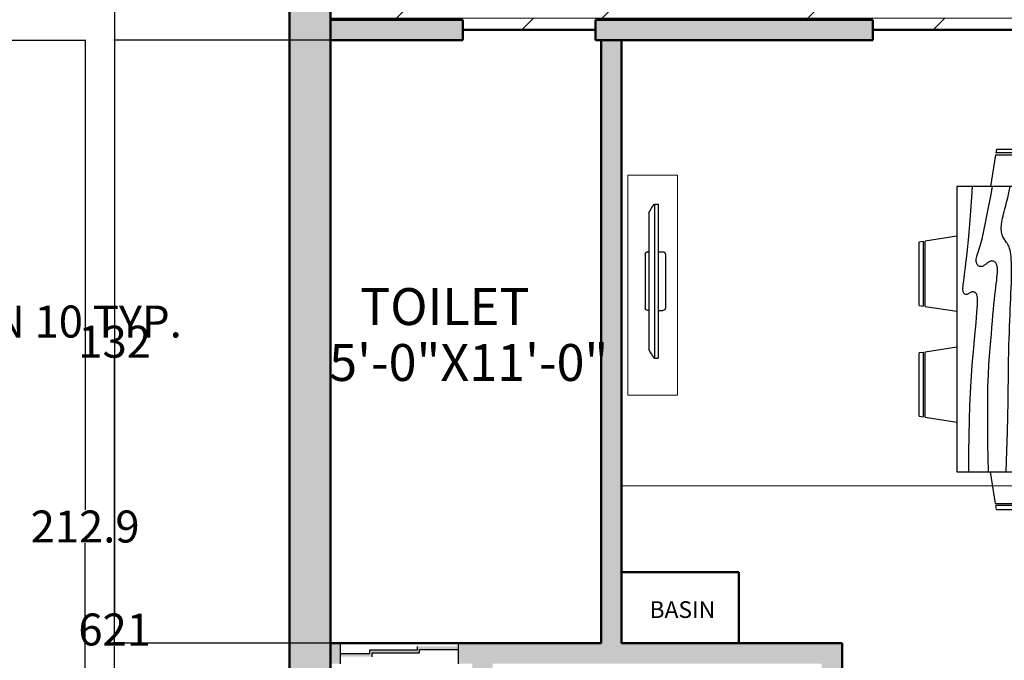
# Model space of a CAD drawing. Units: inches. Extents: x 1381 to 2246, y 1317 to 2168.
# Tile 13 of 15: x 1804 to 2019, y 1776 to 1916. Entities that reach past the tile are written whole.
import ezdxf

# ---------------------------------------------------------------- set-up
doc = ezdxf.new("R2010")
doc.units = ezdxf.units.IN
doc.header["$MEASUREMENT"] = 0
doc.layers.get('0').update_dxf_attribs({"color": 253})
for name, color, linetype, lineweight in [('A-ANNO-DIMS', 2, 'Continuous', 18), ('A-AREA-IDEN', 3, 'Continuous', 25), ('A-FLOR-PATT', 252, 'Continuous', 13), ('A-FURN', 8, 'Continuous', 18), ('A-GLAZ', 4, 'Continuous', 25), ('A-WALL', 7, 'Continuous', 50), ('A-WALL-PATT', 8, 'Continuous', 13)]:
    doc.layers.add(name, color=color, linetype=linetype, lineweight=lineweight)
doc.layers.add('furniture', color=250, linetype='Continuous')
doc.styles.get("Standard").update_dxf_attribs({"font": 'arial.ttf'})
doc.dimstyles.get("Standard").update_dxf_attribs({"dimtxt": 7, "dimasz": 0.18, "dimexe": 0.18, "dimexo": 0.0625, "dimgap": 0.09, "dimtad": 0, "dimtih": 1, "dimtoh": 1, "dimdec": 1, "dimzin": 0, "dimdsep": 46, "dimlunit": 3, "dimtxsty": 'Standard', "dimcen": 0.09, "dimadec": 0, "dimazin": 0, "dimtfac": 1, "dimtdec": 1, "dimtofl": 0, "dimtmove": 0, "dimatfit": 3, "dimfxl": 1, "dimtolj": 1, "dimtzin": 0, "dimarcsym": 0})

# ---------------------------------------------------------------- blocks, each defined once
blk = doc.blocks.new('Dining Set - 36 x 72 in.')
for p, q in [((-22, 27.5), (-22.1562, 26.50042)), ((-22, 27.5), (-6, 27.5)), ((-5.8437, 26.49966), (-6, 27.5)), ((6, 27.5), (5.8438, 26.50042)), ((6, 27.5), (22, 27.5)), ((22.1563, 26.49966), (22, 27.5)), ((-22.2343, 26.00059), (-23.4847, 17.99762)), ((-22.2304, 26), (-5.7608, 26)), ((-5.8416, 26.5), (-22.1534, 26.5)), ((-4.5152, 17.99762), (-5.7655, 25.99926)), ((5.7657, 26.00059), (4.5153, 17.99762)), ((5.7696, 26), (22.2392, 26)), ((22.1584, 26.5), (5.8466, 26.5)), ((23.4848, 17.99762), (22.2345, 25.99926)), ((36, 18), (-36, 18)), ((-36, 18), (-36, -18)), ((36, -18), (36, 18)), ((-45.5, 8), (-44.5004, 8.15617)), ((-45.5, 8), (-45.5, -8)), ((-44.5, -8.15843), (-44.5, 8.15338)), ((-44.0006, 8.23428), (-35.9976, 9.48474)), ((-44, 8.23041), (-44, -8.23915)), ((44.0006, 8.23428), (35.9976, 9.48474)), ((44, 8.23041), (44, -8.23915)), ((44.5, -8.15843), (44.5, 8.15338)), ((45.5, 8), (44.5005, 8.15617)), ((45.5, 8), (45.5, -8)), ((-44.4997, -8.15631), (-45.5, -8)), ((-35.9976, -9.48476), (-43.9993, -8.2345)), ((35.9976, -9.48476), (43.9993, -8.2345)), ((44.4997, -8.15631), (45.5, -8)), ((-36, -18), (36, -18)), ((-22.2343, -26.0006), (-23.4847, -17.99762)), ((-4.5152, -17.99762), (-5.7655, -25.99928)), ((5.7657, -26.0006), (4.5153, -17.99762)), ((23.4848, -17.99762), (22.2345, -25.99928)), ((-22.2304, -26), (-5.7608, -26)), ((-22, -27.5), (-22.1562, -26.50044)), ((-5.8416, -26.5), (-22.1534, -26.5)), ((-5.8437, -26.49967), (-6, -27.5)), ((5.7696, -26), (22.2392, -26)), ((6, -27.5), (5.8438, -26.50044)), ((22.1584, -26.5), (5.8466, -26.5)), ((22.1563, -26.49967), (22, -27.5)), ((-22, -27.5), (-6, -27.5)), ((6, -27.5), (22, -27.5))]:
    blk.add_line(p, q)
for points in [[(-36, 15), (-31.1772, 14.97754), (-26.8079, 14.91406), (-22.8538, 14.81543), (-19.276, 14.6875), (-16.0362, 14.53613), (-13.0957, 14.36718), (-10.4159, 14.18652), (-7.9583, 14), (-5.6904, 13.81315), (-3.6035, 13.63021), (-1.6954, 13.45508), (0.0365, 13.29166), (1.5945, 13.14388), (2.9811, 13.01562), (4.1988, 12.9108), (5.25, 12.83333), (6.1393, 12.78613), (6.8802, 12.76823), (7.4883, 12.77767), (7.9792, 12.8125), (8.3685, 12.87077), (8.6719, 12.95052), (8.9049, 13.0498), (9.0833, 13.16666), (9.2205, 13.29899), (9.3216, 13.44401), (9.3895, 13.59879), (9.4271, 13.76041), (9.4373, 13.92594), (9.4232, 14.09245), (9.3875, 14.257), (9.3333, 14.41666), (9.2638, 14.56917), (9.1836, 14.71484), (9.0975, 14.85465), (9.0104, 14.98958), (8.9272, 15.1206), (8.8529, 15.2487), (8.7922, 15.37483), (8.75, 15.5), (8.7305, 15.62467), (8.7344, 15.74739), (8.7617, 15.86621), (8.8125, 15.97916), (8.8867, 16.08431), (8.9844, 16.17968), (9.1055, 16.26334), (9.25, 16.33333), (9.4189, 16.38802), (9.6172, 16.42708), (9.8506, 16.45052), (10.125, 16.45833), (10.4463, 16.45052), (10.8203, 16.42708), (11.2529, 16.38802), (11.75, 16.33333), (12.3184, 16.26318), (12.9694, 16.17838), (13.7151, 16.07991), (14.5677, 15.96875), (15.5395, 15.84586), (16.6426, 15.71224), (17.8893, 15.56884), (19.2917, 15.41666), (20.859, 15.25667), (22.5879, 15.08984), (24.4721, 14.91715), (26.5052, 14.73958), (28.6809, 14.5581), (30.9929, 14.3737), (33.4347, 14.18733), (36, 14)], [(-36, 10), (-28.9766, 10.14274), (-23.1725, 10.20442), (-18.4241, 10.19775), (-14.5677, 10.13541), (-11.4399, 10.03011), (-8.877, 9.89453), (-6.7154, 9.74137), (-4.7917, 9.58333), (-2.9698, 9.43082), (-1.2246, 9.28515), (0.4415, 9.14534), (2.026, 9.01041), (3.5266, 8.87939), (4.9408, 8.7513), (6.266, 8.62516), (7.5, 8.5), (8.6411, 8.37549), (9.6914, 8.2539), (10.6538, 8.13818), (11.5312, 8.03125), (12.3267, 7.93603), (13.043, 7.85547), (13.6831, 7.79248), (14.25, 7.75), (14.7471, 7.7303), (15.1797, 7.73307), (15.5537, 7.75732), (15.875, 7.80208), (16.1494, 7.86637), (16.3828, 7.94922), (16.5811, 8.04964), (16.75, 8.16666), (16.8944, 8.29915), (17.0143, 8.44531), (17.1089, 8.60319), (17.1771, 8.77083), (17.218, 8.94629), (17.2305, 9.1276), (17.2137, 9.31282), (17.1667, 9.5), (17.0895, 9.6875), (16.987, 9.875), (16.8649, 10.0625), (16.7292, 10.25), (16.5856, 10.4375), (16.4401, 10.625), (16.2985, 10.8125), (16.1667, 11), (16.05, 11.18733), (15.9518, 11.3737), (15.8752, 11.5581), (15.8229, 11.73958), (15.798, 11.91715), (15.8034, 12.08984), (15.842, 12.25667), (15.9167, 12.41666), (16.0295, 12.56836), (16.1784, 12.70833), (16.3605, 12.83268), (16.5729, 12.9375), (16.8127, 13.01888), (17.0768, 13.07291), (17.3625, 13.0957), (17.6667, 13.08333), (17.9894, 13.03312), (18.3418, 12.94726), (18.7382, 12.82918), (19.1927, 12.68229), (19.7195, 12.51001), (20.3327, 12.31575), (21.0465, 12.10294), (21.875, 11.875), (22.8357, 11.63354), (23.959, 11.37304), (25.2786, 11.08618), (26.8282, 10.76562), (28.6414, 10.40405), (30.752, 9.99414), (33.1936, 9.52856), (36, 9)], [(-36, 5.5), (-30.7157, 5.3348), (-26.069, 5.20963), (-21.9946, 5.11767), (-18.4271, 5.05208), (-15.3009, 5.00602), (-12.5508, 4.97265), (-10.1112, 4.94515), (-7.9167, 4.91666), (-5.909, 4.88167), (-4.0586, 4.83984), (-2.3429, 4.79215), (-0.7396, 4.73958), (0.7739, 4.6831), (2.22, 4.6237), (3.6213, 4.56233), (5, 4.5), (6.373, 4.43782), (7.7344, 4.3776), (9.0723, 4.32129), (10.375, 4.27083), (11.6309, 4.22819), (12.8281, 4.19531), (13.9551, 4.17415), (15, 4.16666), (15.954, 4.17448), (16.819, 4.19791), (17.6001, 4.23698), (18.3021, 4.29166), (18.9299, 4.36198), (19.4883, 4.44791), (19.9823, 4.54948), (20.4167, 4.66666), (20.7969, 4.79899), (21.1302, 4.94401), (21.4245, 5.09879), (21.6875, 5.26041), (21.9271, 5.42594), (22.1511, 5.59245), (22.3672, 5.757), (22.5834, 5.91666), (22.8065, 6.06868), (23.0404, 6.21093), (23.2879, 6.34147), (23.5521, 6.45833), (23.8358, 6.55957), (24.142, 6.64323), (24.4735, 6.70735), (24.8334, 6.75), (25.2235, 6.76969), (25.642, 6.76692), (26.0858, 6.74267), (26.5521, 6.69791), (27.0379, 6.63362), (27.5404, 6.55078), (28.0565, 6.45036), (28.5834, 6.33333), (29.1242, 6.19987), (29.7071, 6.04687), (30.3661, 5.87044), (31.1354, 5.66666), (32.0493, 5.43164), (33.142, 5.16146), (34.4475, 4.85221), (36, 4.5)], [(-36, -1), (-30.7915, -0.6591), (-26.0195, -0.38216), (-21.6519, -0.16284), (-17.6563, 0.00521), (-14.0005, 0.12833), (-10.6523, 0.21289), (-7.5796, 0.26522), (-4.75, 0.29166), (-2.134, 0.29793), (0.2878, 0.28711), (2.5317, 0.26163), (4.6146, 0.22396), (6.5529, 0.17651), (8.3633, 0.12174), (10.0623, 0.06209), (11.6667, 0), (13.1899, -0.06201), (14.6341, -0.1211), (15.9982, -0.17432), (17.2813, -0.21875), (18.4823, -0.25147), (19.6003, -0.26953), (20.6343, -0.27002), (21.5834, -0.25), (22.4481, -0.20768), (23.2357, -0.14584), (23.9549, -0.06836), (24.6146, 0.02083), (25.2235, 0.11784), (25.7904, 0.21875), (26.3241, 0.31966), (26.8334, 0.41666), (27.3265, 0.50618), (27.8099, 0.58593), (28.2894, 0.65397), (28.7709, 0.70833), (29.2601, 0.74707), (29.763, 0.76823), (30.2855, 0.76985), (30.8334, 0.75), (31.4088, 0.70784), (31.9994, 0.64713), (32.589, 0.57275), (33.1615, 0.48958), (33.7008, 0.4025), (34.1908, 0.3164), (34.6153, 0.23616), (34.9584, 0.16666), (35.2099, 0.11165), (35.3848, 0.07031), (35.504, 0.04069), (35.5886, 0.02083), (35.6594, 0.00879), (35.7377, 0.0026), (35.8442, 0.00032), (36, 0)], [(-36, -6.5), (-27.1843, -6.31267), (-20.084, -6.1263), (-14.469, -5.9419), (-10.1094, -5.76042), (-6.7752, -5.58285), (-4.2363, -5.41016), (-2.2629, -5.24333), (-0.625, -5.08334), (0.8708, -4.93099), (2.2715, -4.78646), (3.5872, -4.64974), (4.8281, -4.52084), (6.0046, -4.39974), (7.127, -4.28646), (8.2053, -4.18099), (9.25, -4.08334), (10.2705, -3.99382), (11.2734, -3.91407), (12.2647, -3.84603), (13.25, -3.79167), (14.2354, -3.75293), (15.2266, -3.73177), (16.2295, -3.73015), (17.25, -3.75), (18.2912, -3.79248), (19.3451, -3.85547), (20.4009, -3.93604), (21.4479, -4.03125), (22.4754, -4.13819), (23.4727, -4.25391), (24.4289, -4.37549), (25.3334, -4.5), (26.1785, -4.62492), (26.9694, -4.74935), (27.7145, -4.87281), (28.4219, -4.99479), (29.1, -5.11483), (29.7572, -5.23242), (30.4016, -5.34709), (31.0417, -5.45834), (31.6837, -5.56437), (32.3262, -5.65821), (32.9658, -5.73153), (33.599, -5.77604), (34.2224, -5.78345), (34.8327, -5.74545), (35.4264, -5.65373), (36, -5.5)], [(-36, -10), (-26.4022, -9.81299), (-18.4675, -9.62891), (-11.9839, -9.45069), (-6.7396, -9.28125), (-2.5226, -9.12354), (0.8789, -8.98047), (3.6769, -8.85498), (6.0833, -8.75), (8.2767, -8.66765), (10.3021, -8.60677), (12.1712, -8.56543), (13.8958, -8.54167), (15.4876, -8.53353), (16.9583, -8.53907), (18.3197, -8.55632), (19.5834, -8.58334), (20.7616, -8.61841), (21.8685, -8.66081), (22.9188, -8.71004), (23.9271, -8.76563), (24.9081, -8.82707), (25.8763, -8.89388), (26.8465, -8.96558), (27.8334, -9.04167), (28.8474, -9.12118), (29.8828, -9.20117), (30.93, -9.27824), (31.9792, -9.34896), (33.0205, -9.40991), (34.0443, -9.45768), (35.0407, -9.48885), (36, -9.5)], [(-36, -14.5), (-30.0881, -14.33513), (-25.0332, -14.21224), (-20.7312, -14.12647), (-17.0781, -14.07292), (-13.97, -14.04671), (-11.3027, -14.04297), (-8.9724, -14.05681), (-6.875, -14.08334), (-4.9224, -14.11833), (-3.0905, -14.16016), (-1.3709, -14.20785), (0.2448, -14.26042), (1.7647, -14.3169), (3.1973, -14.3763), (4.5507, -14.43767), (5.8333, -14.5), (7.0554, -14.5621), (8.235, -14.62175), (9.3922, -14.67652), (10.5469, -14.72396), (11.7192, -14.76164), (12.929, -14.78711), (14.1965, -14.79794), (15.5417, -14.79167), (16.9933, -14.76424), (18.6152, -14.70508), (20.4804, -14.60197), (22.6615, -14.44271), (25.2312, -14.21509), (28.2624, -13.9069), (31.8277, -13.50594), (36, -13)]]:
    blk.add_lwpolyline(points)
blk = doc.blocks.new('dining area')
at = {"layer": 'furniture', "xscale": 0.6659924291999282, "yscale": 0.6659924291999282, "zscale": 0.6659924291999282, "rotation": 90}
blk.add_blockref('Dining Set - 36 x 72 in.', (-0.44, 20.51), dxfattribs=at)
blk = doc.blocks.new('PLASMA-LARGE')
at = {"layer": 'furniture'}
for p, q in [((-7.26, 0), (7.26, 0)), ((-21, -2.5), (21, -2.5)), ((-21, -2.5), (-21, -3.5)), ((-18.61, -1), (18.61, -1)), ((-8, -1), (-8, -0.74)), ((8, -1), (8, -0.74)), ((21, -2.5), (21, -3.5)), ((-21, -3.5), (21, -3.5)), ((-8, -3.5), (-8, -4.76)), ((8, -3.5), (8, -4.76)), ((-7.26, -5.5), (7.26, -5.5))]:
    blk.add_line(p, q, dxfattribs=at)
for centre, radius, start, end in [((-7.26, -0.74), 0.744, 90, 180), ((7.26, -0.74), 0.744, 0, 90), ((-13.97, -11.05), 11.07, 114.7602, 129.4175), ((13.97, -11.05), 11.07, 50.5825, 65.2398), ((-7.26, -4.76), 0.744, 180, 270), ((7.26, -4.76), 0.744, 270, 0)]:
    blk.add_arc(centre, radius, start, end, dxfattribs=at)
blk = doc.blocks.new('CONSOLE')
for p, q in [((10.82, 48.12), (0, 48.12)), ((0, 48.12), (0, 0)), ((10.82, 0), (10.82, 48.12)), ((0, 0), (10.82, 0))]:
    blk.add_line(p, q)
blk = doc.blocks.new('*D25')
at = {"layer": 'A-ANNO-DIMS', "color": 0, "lineweight": -2, "transparency": 16777216}
for p, q in [((1721.71, 1848.36), (1721.71, 1850.02)), ((1721.89, 1849.84), (1731.83, 1849.84)), ((1732.01, 1848.36), (1732.01, 1850.02)), ((1732.01, 1849.84), (1732.19, 1849.84))]:
    blk.add_line(p, q, dxfattribs=at)
at = {"layer": 'A-ANNO-DIMS', "color": 0, "transparency": 16777216}
for points in [[(1721.89, 1849.87), (1721.89, 1849.81), (1721.71, 1849.84)], [(1731.83, 1849.87), (1731.83, 1849.81), (1732.01, 1849.84)]]:
    blk.add_solid(points, dxfattribs=at)
at = {"layer": 'Defpoints', "color": 0, "transparency": 16777216}
for p in [(1732.01, 1849.84), (1721.71, 1848.3), (1732.01, 1848.3)]:
    blk.add_point(p, dxfattribs=at)
at = {"layer": 'A-ANNO-DIMS', "color": 0, "transparency": 16777216, "insert": (1787.87, 1849.84), "char_height": 7, "attachment_point": 5}
blk.add_mtext('\\A1;SOFA CUSHION 10 TYP.', dxfattribs=at)
blk = doc.blocks.new('*D61')
at = {"layer": 'A-ANNO-DIMS', "color": 0, "lineweight": -2, "transparency": 16777216}
for p, q in [((1737.61, 1911.42), (1818.27, 1911.42)), ((1818.09, 1911.24), (1818.09, 1808.63)), ((1818.09, 1698.7), (1818.09, 1801.3)), ((1737.61, 1698.52), (1818.27, 1698.52))]:
    blk.add_line(p, q, dxfattribs=at)
at = {"layer": 'A-ANNO-DIMS', "color": 0, "transparency": 16777216}
for points in [[(1818.06, 1911.24), (1818.12, 1911.24), (1818.09, 1911.42)], [(1818.06, 1698.7), (1818.12, 1698.7), (1818.09, 1698.52)]]:
    blk.add_solid(points, dxfattribs=at)
at = {"layer": 'Defpoints', "color": 0, "transparency": 16777216}
for p in [(1737.55, 1911.42), (1818.09, 1911.42), (1737.55, 1698.52)]:
    blk.add_point(p, dxfattribs=at)
at = {"layer": 'A-ANNO-DIMS', "color": 0, "transparency": 16777216, "insert": (1818.09, 1804.97), "char_height": 7, "attachment_point": 5}
blk.add_mtext('\\A1;212.9', dxfattribs=at)
blk = doc.blocks.new('*D76')
at = {"layer": 'A-ANNO-DIMS', "color": 0, "lineweight": -2, "transparency": 16777216}
for p, q in [((1862.74, 2092.92), (1824.38, 2092.92)), ((1824.56, 2092.74), (1824.56, 1786.08)), ((1824.56, 1472.1), (1824.56, 1778.75)), ((1862.74, 1471.92), (1824.38, 1471.92))]:
    blk.add_line(p, q, dxfattribs=at)
at = {"layer": 'A-ANNO-DIMS', "color": 0, "transparency": 16777216}
for points in [[(1824.53, 2092.74), (1824.59, 2092.74), (1824.56, 2092.92)], [(1824.53, 1472.1), (1824.59, 1472.1), (1824.56, 1471.92)]]:
    blk.add_solid(points, dxfattribs=at)
at = {"layer": 'Defpoints', "color": 0, "transparency": 16777216}
for p in [(1824.56, 2092.92), (1862.81, 2092.92), (1862.81, 1471.92)]:
    blk.add_point(p, dxfattribs=at)
at = {"layer": 'A-ANNO-DIMS', "color": 0, "transparency": 16777216, "insert": (1824.56, 1782.42), "char_height": 7, "attachment_point": 5}
blk.add_mtext('\\A1;621', dxfattribs=at)
blk = doc.blocks.new('*D82')
at = {"layer": 'A-ANNO-DIMS', "color": 0, "lineweight": -2, "transparency": 16777216}
for p, q in [((1871.74, 1911.42), (1824.38, 1911.42)), ((1824.56, 1911.24), (1824.56, 1849.08)), ((1824.56, 1779.6), (1824.56, 1841.75)), ((1871.74, 1779.42), (1824.38, 1779.42))]:
    blk.add_line(p, q, dxfattribs=at)
at = {"layer": 'A-ANNO-DIMS', "color": 0, "transparency": 16777216}
for points in [[(1824.53, 1911.24), (1824.59, 1911.24), (1824.56, 1911.42)], [(1824.53, 1779.6), (1824.59, 1779.6), (1824.56, 1779.42)]]:
    blk.add_solid(points, dxfattribs=at)
at = {"layer": 'Defpoints', "color": 0, "transparency": 16777216}
for p in [(1824.56, 1911.42), (1871.81, 1911.42), (1871.81, 1779.42)]:
    blk.add_point(p, dxfattribs=at)
at = {"layer": 'A-ANNO-DIMS', "color": 0, "transparency": 16777216, "insert": (1824.56, 1845.42), "char_height": 7, "attachment_point": 5}
blk.add_mtext('\\A1;132', dxfattribs=at)

msp = doc.modelspace()

# ---------------------------------------------------------------- hatches: boundary and pattern name
at = {"layer": 'A-FLOR-PATT'}
h = msp.add_hatch(dxfattribs=at)
h.set_pattern_fill('DOLMIT', color=256, scale=15)
h.paths.add_polyline_path([(2033.8052, 2083.9163), (1932.8359, 2083.9163), (1932.8359, 2057.4148), (1871.8052, 2057.4148), (1871.8052, 1915.9163), (1900.7902, 1915.9163), (1900.7902, 1913.6663), (1929.807, 1913.6663), (1929.807, 1915.9163), (1990.4785, 1915.9163), (1990.4785, 1913.6663), (2028.7731, 1913.6663), (2028.7731, 1915.9163), (2033.8052, 1915.9163)])
edge = h.paths.add_edge_path(flags=16)
edge.add_spline(control_points=[(1939.5401, 1955.9789), (1939.5923, 1955.9054), (1939.7074, 1955.7434), (1939.52, 1955.4418), (1939.2609, 1955.0703), (1939.5201, 1954.8623), (1939.6513, 1954.757)], knot_values=[0, 0, 0, 0, 0.37399428, 0.82431366, 1.46117297, 2.11445126, 2.11445126, 2.11445126, 2.11445126], degree=3, periodic=0)
edge.add_spline(control_points=[(1939.8748, 1955.9789), (1939.9271, 1955.9054), (1940.0422, 1955.7434), (1939.8548, 1955.4418), (1939.5956, 1955.0703), (1939.8548, 1954.8623), (1939.986, 1954.757)], knot_values=[0, 0, 0, 0, 0.37399428, 0.82431366, 1.46117297, 2.11445126, 2.11445126, 2.11445126, 2.11445126], degree=3, periodic=0)
edge = h.paths.add_edge_path(flags=16)
edge.add_line((1942.0171, 2024.4608), (1942.0171, 1955.9789))
edge.add_line((1942.0171, 1955.9789), (1913.4617, 1955.9789))
edge.add_line((1913.4617, 1955.9789), (1913.4617, 1962.7697))
edge.add_line((1913.4617, 1962.7697), (1887.334, 1962.7697))
edge.add_line((1887.334, 1962.7697), (1887.445, 1951.263))
edge.add_line((1887.445, 1951.263), (1874.2492, 1951.263))
edge.add_line((1874.2492, 1951.263), (1874.1382, 1962.7697))
edge.add_line((1874.1382, 1962.7697), (1874.1382, 2014.1291))
edge.add_line((1874.1382, 2014.1291), (1874.0273, 2025.6358))
edge.add_line((1874.0273, 2025.6358), (1887.2231, 2025.6358))
edge.add_line((1887.2231, 2025.6358), (1887.334, 2014.1291))
edge.add_line((1887.334, 2014.1291), (1913.4617, 2014.1291))
edge.add_line((1913.4617, 2014.1291), (1913.4617, 2024.4608))
edge.add_line((1913.4617, 2024.4608), (1939.579, 2024.4608))
edge.add_spline(control_points=[(1939.579, 2024.4608), (1939.6269, 2024.5305), (1939.736, 2024.6891), (1939.5499, 2024.9858), (1939.2914, 2025.3575), (1939.5505, 2025.5655), (1939.6817, 2025.6708)], knot_values=[0, 0, 0, 0, 0.3521435, 0.80246288, 1.43932219, 2.09260048, 2.09260048, 2.09260048, 2.09260048], degree=3, periodic=0)
edge.add_spline(control_points=[(1940.0164, 2025.6708), (1939.8852, 2025.5655), (1939.6261, 2025.3575), (1939.8847, 2024.9858), (1940.0707, 2024.6891), (1939.9616, 2024.5305), (1939.9137, 2024.4608)], knot_values=[0, 0, 0, 0, 0.65327829, 1.2901376, 1.74045698, 2.09260048, 2.09260048, 2.09260048, 2.09260048], degree=3, periodic=0)
edge.add_line((1939.9137, 2024.4608), (1942.0171, 2024.4608))
h.paths.add_polyline_path([(1891.698, 2014.0737), (1891.698, 2004.8072), (1884.8656, 2004.8072), (1884.8197, 2004.7449), (1884.8197, 1968.5691), (1877.0588, 1968.5691), (1877.0588, 1983.6181), (1884.8197, 1983.6181), (1884.8197, 1989.7582), (1877.0588, 1989.7582), (1877.0588, 2004.8072), (1884.8656, 2004.8072)], flags=0)
h.paths.add_polyline_path([(1884.8729, 2020.1923, -1), (1876.3774, 2020.1923, -1)], flags=0)
h.paths.add_polyline_path([(1884.9838, 1957.3262, -1), (1876.4884, 1957.3262, -1)], flags=0)
h.paths.add_polyline_path([(1949.3287, 1985.8776), (2018.4467, 1985.8776), (2018.4467, 1998.2538), (1949.3287, 1998.2538)], flags=24)
h.paths.add_polyline_path([(1951.1032, 2002.3157), (2019.8384, 2002.3157), (2019.8384, 2014.8488), (1951.1032, 2014.8488)], flags=24)
at = {"layer": 'A-GLAZ'}
h = msp.add_hatch(color=256, dxfattribs=at)
h.dxf.hatch_style = 1
h.paths.add_polyline_path([(1880.8856, 1777.3422), (1891.2803, 1777.3422), (1891.2803, 1778.0682), (1899.8394, 1778.0682), (1899.8394, 1778.7283), (1890.8398, 1778.7283), (1890.8398, 1777.9582), (1880.4011, 1777.9582), (1880.4011, 1777.1663), (1873.9195, 1777.1663), (1873.9195, 1776.4401), (1880.8856, 1776.4401)])
at = {"layer": 'A-WALL-PATT'}
h = msp.add_hatch(color=256, dxfattribs=at)
h.dxf.hatch_style = 1
h.paths.add_polyline_path([(1990.4785, 1915.9163), (1929.807, 1915.9163), (1929.807, 1911.4163), (1990.4785, 1911.4163)], flags=17)
h.paths.add_polyline_path([(1900.7902, 1915.9163), (1871.8052, 1915.9163), (1871.8052, 1911.4163), (1900.7902, 1911.4163)], flags=17)
h.paths.add_polyline_path([(2043.2216, 1915.9163), (2038.3052, 1915.9163), (2038.3052, 2035.4163), (2098.0373, 2035.4163), (2098.0373, 2039.9163), (2033.8052, 2039.9163), (2033.8052, 1915.9163), (2028.7731, 1915.9163), (2028.7731, 1911.4163), (2043.2216, 1911.4163)], flags=17)
h.paths.add_polyline_path([(2153.3052, 1915.9163), (2085.2216, 1915.9163), (2085.2216, 1911.4163), (2153.3052, 1911.4163)], flags=17)
h.paths.add_polyline_path([(1935.508, 1911.4163), (1931.008, 1911.4163), (1931.008, 1779.4163), (1899.8394, 1779.4163), (1899.8394, 1774.9163), (1902.8052, 1774.9163), (1979.3052, 1774.9163), (1979.3052, 1770.3401), (1983.8052, 1770.3401), (1983.8052, 1779.4163), (1935.508, 1779.4163)], flags=17)
h.paths.add_polyline_path([(1871.8052, 2083.9163), (2153.3052, 2083.9163), (2153.3052, 2039.9163), (2141.7178, 2039.9163), (2141.7178, 2035.4163), (2153.3052, 2035.4163), (2153.3052, 1471.9163), (2162.3052, 1471.9163), (2162.3052, 2092.9163), (1862.8052, 2092.9163), (1862.8052, 1471.9163), (1904.4174, 1471.9163), (1904.4174, 1480.9163), (1871.8052, 1480.9163), (1871.8052, 1569.4163), (1964.2348, 1569.4163), (1964.2348, 1578.4163), (1871.8052, 1578.4163)])
h.paths.add_polyline_path([(1907.3052, 1729.193), (1902.8052, 1729.193), (1902.8052, 1714.9163), (1871.8052, 1714.9163), (1871.8052, 1710.4163), (1932.8736, 1710.4163), (1932.8736, 1714.9163), (1907.3052, 1714.9163)], flags=17)
h.paths.add_polyline_path([(2044.3052, 1644.4163), (2039.8052, 1644.4163), (2039.8052, 1618.2205), (2044.3052, 1618.2205)], flags=17)
h.paths.add_polyline_path([(2044.3052, 1581.7679), (2039.8052, 1581.7679), (2039.8052, 1578.4163), (2027.577, 1578.4163), (2027.577, 1569.4163), (2044.3052, 1569.4163)], flags=17)
h = msp.add_hatch(color=256, dxfattribs=at)
h.dxf.hatch_style = 1
h.paths.add_polyline_path([(1873.9195, 1779.4163), (1871.8052, 1779.4163), (1871.8052, 1774.9163), (1873.9195, 1774.9163)])
h.paths.add_polyline_path([(1983.8052, 1779.4163), (1935.508, 1779.4163), (1935.508, 1911.4163), (1931.008, 1911.4163), (1931.008, 1779.4163), (1899.8394, 1779.4163), (1899.8394, 1774.9163), (1902.8052, 1774.9163), (1979.3052, 1774.9163), (1979.3052, 1770.3401), (1983.8052, 1770.3401)])
h.paths.add_polyline_path([(1907.3052, 1774.9163), (1902.8052, 1774.9163), (1902.8052, 1755.1129), (1907.3052, 1755.1129)])
h.paths.add_polyline_path([(1983.8052, 1734.7997), (1979.3052, 1734.7997), (1979.3052, 1714.9163), (1973.3503, 1714.9163), (1973.3503, 1710.4163), (1983.8052, 1710.4163)])
h.paths.add_polyline_path([(2044.3052, 1732.454), (2039.8052, 1732.454), (2039.8052, 1716.0149), (2024.8052, 1716.0149), (2024.8052, 1710.4163), (2039.8052, 1710.4163), (2039.8052, 1644.4163), (2044.3052, 1644.4163)])
h.paths.add_polyline_path([(2056.2659, 1677.4163), (2044.3052, 1677.4163), (2044.3052, 1672.9163), (2056.2659, 1672.9163)])
h.paths.add_polyline_path([(2119.6192, 1677.4163), (2104.2659, 1677.4163), (2104.2659, 1672.9163), (2119.6192, 1672.9163)])
h.paths.add_polyline_path([(2012.5552, 1480.9163), (1952.401, 1480.9163), (1952.401, 1471.9163), (2012.5552, 1471.9163)])
h.paths.add_polyline_path([(1870.8149, 1834.6368), (1933.6567, 1834.6368), (1933.6567, 1847.0047), (1870.8149, 1847.0047)], flags=9)

# ---------------------------------------------------------------- linework, layer by layer
at = {"layer": 'A-ANNO-DIMS'}
msp.add_line((1935.508, 1813.9071), (2153.3052, 1813.9071), dxfattribs=at)
at = {"layer": 'A-GLAZ'}
for p, q in [((1873.9195, 1779.4163), (1873.9195, 1774.9163)), ((1899.8394, 1779.4163), (1873.9195, 1779.4163)), ((1880.4011, 1777.1663), (1880.4011, 1777.9582)), ((1880.4011, 1777.9582), (1890.8398, 1777.9582)), ((1890.8398, 1777.9582), (1890.8398, 1778.7283)), ((1891.2803, 1777.3422), (1891.2803, 1778.0682)), ((1891.2803, 1778.0682), (1899.8394, 1778.0682)), ((1899.8394, 1774.9163), (1899.8394, 1779.4163)), ((1873.9195, 1777.1663), (1880.4011, 1777.1663)), ((1880.8856, 1776.4401), (1880.8856, 1777.3422)), ((1880.8856, 1777.3422), (1891.2803, 1777.3422))]:
    msp.add_line(p, q, dxfattribs=at)
at = {"layer": 'A-WALL'}
for p, q in [((1862.8052, 2092.9163), (1862.8052, 1471.9163)), ((1871.8052, 2083.9163), (1871.8052, 1578.4163)), ((1871.8052, 1915.9163), (1900.7902, 1915.9163)), ((1900.7902, 1915.9163), (1900.7902, 1911.4163)), ((1929.807, 1915.9163), (1929.807, 1911.4163)), ((1929.807, 1915.9163), (1990.4785, 1915.9163)), ((1990.4785, 1915.9163), (1990.4785, 1911.4163)), ((1900.7902, 1913.6663), (1929.807, 1913.6663)), ((1990.4785, 1913.6663), (2028.7731, 1913.6663)), ((1871.8052, 1911.4163), (1900.7902, 1911.4163)), ((1929.807, 1911.4163), (1990.4785, 1911.4163)), ((1931.008, 1911.4163), (1931.008, 1779.4163)), ((1935.508, 1911.4163), (1935.508, 1779.4163)), ((1935.508, 1794.9885), (1961.1337, 1794.9885)), ((1961.1337, 1794.9885), (1961.1337, 1779.4163)), ((1871.8052, 1779.4163), (1931.008, 1779.4163)), ((1935.508, 1779.4163), (1983.8052, 1779.4163)), ((1983.8052, 1779.4163), (1983.8052, 1770.3401))]:
    msp.add_line(p, q, dxfattribs=at)

# ---------------------------------------------------------------- block references
at = {"layer": 'A-FURN', "xscale": 1.301533394022331, "yscale": 1.301533394022331, "zscale": 1.301533394022331}
msp.add_blockref('dining area', (2025.0396, 1821.4677), dxfattribs=at)
at = {"layer": 'A-FURN', "rotation": 180}
msp.add_blockref('CONSOLE', (1947.7221, 1881.8498), dxfattribs=at)
at = {"layer": 'A-FURN', "xscale": -0.8031214548296134, "yscale": 0.8031214548296134, "zscale": 0.8031214548296134, "rotation": 90}
msp.add_blockref('PLASMA-LARGE', (1940.6826, 1858.6869), dxfattribs=at)

# ---------------------------------------------------------------- texts
at = {"layer": 'A-AREA-IDEN'}
for s, height, p in [('TOILET', 8.07451, (1878.2702, 1849.0755)), ('5\'-0"X11\'-0"', 8.074511, (1871.5107, 1836.8359)), ('BASIN', 3.66027, (1941.6231, 1784.9463))]:
    msp.add_text(s, height=height, dxfattribs=at).set_placement(p)

# ---------------------------------------------------------------- dimensions: what is measured, and where the dimension line sits
at = {"layer": 'A-ANNO-DIMS'}
for base, p1, p2, override, picture, middle in [((1824.5552, 2092.9163), (1862.8052, 1471.9163), (1862.8052, 2092.9163), {"dimdec": 0, "dimlfac": 1, "dimrnd": 0, "dimzin": 0, "dimdsep": 46, "dimlunit": 2}, '*D76', (1824.5552, 1782.4163)), ((1818.0904, 1911.4163), (1737.551, 1698.5169), (1737.551, 1911.4163), {"dimdec": 1, "dimlfac": 1, "dimrnd": 0, "dimzin": 0, "dimdsep": 46, "dimlunit": 2}, '*D61', (1818.0904, 1804.9666)), ((1824.5552, 1911.4163), (1871.8052, 1779.4163), (1871.8052, 1911.4163), {"dimdec": 0, "dimlfac": 1, "dimrnd": 0, "dimzin": 0, "dimdsep": 46, "dimlunit": 2}, '*D82', (1824.5552, 1845.4163))]:
    dim = msp.add_linear_dim(base=base, p1=p1, p2=p2, angle=90, dimstyle='Standard', override=override, dxfattribs=at)
    dim.commit()
    dim.dimension.update_dxf_attribs({"geometry": picture, "text_midpoint": middle})
dim = msp.add_linear_dim(base=(1732.0082, 1849.8418), p1=(1721.7081, 1848.2968), p2=(1732.0082, 1848.2968), text='SOFA CUSHION <> TYP.', dimstyle='Standard', override={"dimdec": 0, "dimrnd": 0, "dimzin": 0, "dimlunit": 2}, dxfattribs=at)
dim.commit()
dim.dimension.update_dxf_attribs({"geometry": '*D25', "text_midpoint": (1787.8747, 1849.8418)})

doc.saveas('drawing.dxf')
